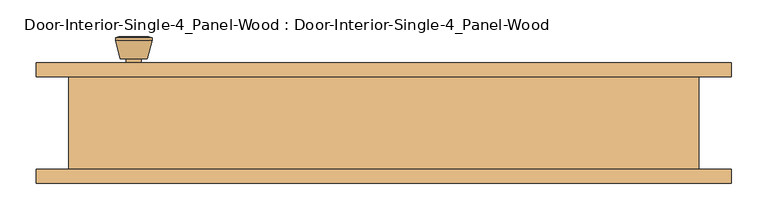
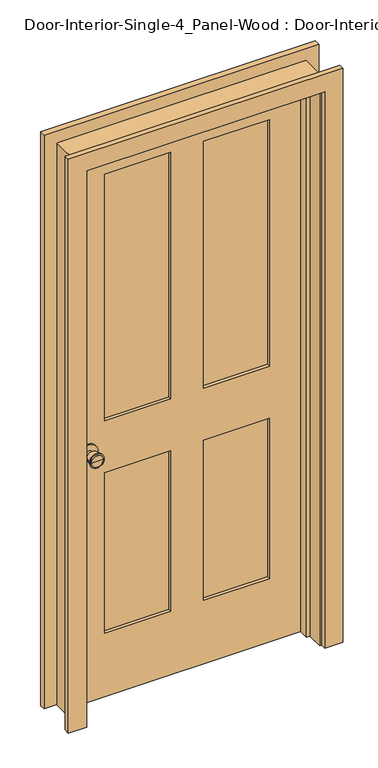
"""IFC4 building model written with IfcOpenShell, lengths in millimetres: door geometry, Door-Interior-Single-4_Panel-Wood : Door-Interior-Single-4_Panel-Wood."""

from ifc_helpers import new_model, si_unit, point, frame, frame_2d, origin, place, context, project, spatial, polyline, circle_curve, trimmed, segment, composite_curve, outline, extrude, faceted_brep, source, transform, mapped, element, save
from ifc_brep_helpers import plane_surface, cylinder_surface, revolved_surface, advanced_brep


def door_interior_single_4_panel_wood_door_interior_single_4_d89ef9d3(model_context):
    return source(origin(), model_context, "Body", "SolidModel", [
        advanced_brep(
        [(-342.9, 19.4, 914.4), (-332.9, 19.4, 914.4), (-352.9, 19.4, 914.4), (-322.4241324, -29.6, 914.4), (-342.9, -29.6, 914.4), (-363.3758676, -29.6, 914.4), (-317.9, -27.7721319, 914.4), (-367.9, -27.7721319, 914.4), (-317.9, -24.3084537, 914.4), (-367.9, -24.3084537, 914.4), (-324.263764, 0.4, 914.4), (-361.536236, 0.4, 914.4), (-332.9, 0.4, 914.4), (-352.9, 0.4, 914.4)],
        [
            (0, 1),
            (1, 2, circle_curve(frame((-342.9, 19.4, 914.4), z_axis=(0.0, 1.0, 0.0), x_axis=(-1.0, 0.0, 0.0)), 10.0)),
            (2, 0),
            (2, 1, circle_curve(frame((-342.9, 19.4, 914.4), z_axis=(0.0, 1.0, 0.0), x_axis=(-1.0, 0.0, 0.0)), 10.0)),
            (3, 4),
            (4, 5),
            (5, 3, circle_curve(frame((-342.9, -29.6, 914.4), z_axis=(0.0, -1.0, 0.0), x_axis=(-1.0, 0.0, 0.0)), 20.4758676)),
            (3, 5, circle_curve(frame((-342.9, -29.6, 914.4), z_axis=(0.0, -1.0, 0.0), x_axis=(-1.0, 0.0, 0.0)), 20.4758676)),
            (6, 3),
            (5, 7),
            (7, 6, circle_curve(frame((-342.9, -27.7721319, 914.4), z_axis=(0.0, -1.0, 0.0), x_axis=(-1.0, 0.0, 0.0)), 25.0)),
            (6, 7, circle_curve(frame((-342.9, -27.7721319, 914.4), z_axis=(0.0, -1.0, 0.0), x_axis=(-1.0, 0.0, 0.0)), 25.0)),
            (8, 6),
            (7, 9),
            (9, 8, circle_curve(frame((-342.9, -24.3084537, 914.4), z_axis=(0.0, -1.0, 0.0), x_axis=(-1.0, 0.0, 0.0)), 25.0)),
            (8, 9, circle_curve(frame((-342.9, -24.3084537, 914.4), z_axis=(0.0, -1.0, 0.0), x_axis=(-1.0, 0.0, 0.0)), 25.0)),
            (10, 8),
            (9, 11),
            (11, 10, circle_curve(frame((-342.9, 0.4, 914.4), z_axis=(0.0, -1.0, 0.0), x_axis=(-1.0, 0.0, 0.0)), 18.636236)),
            (10, 11, circle_curve(frame((-342.9, 0.4, 914.4), z_axis=(0.0, -1.0, 0.0), x_axis=(-1.0, 0.0, 0.0)), 18.636236)),
            (12, 10),
            (11, 13),
            (13, 12, circle_curve(frame((-342.9, 0.4, 914.4), z_axis=(0.0, -1.0, 0.0), x_axis=(-1.0, 0.0, 0.0)), 10.0)),
            (12, 13, circle_curve(frame((-342.9, 0.4, 914.4), z_axis=(0.0, -1.0, 0.0), x_axis=(-1.0, 0.0, 0.0)), 10.0)),
            (1, 12),
            (13, 2),
        ],
        [
            plane_surface(frame((-342.9, 19.4, 914.4), z_axis=(0.0, 1.0, 0.0), x_axis=(-1.0, 0.0, 0.0))),
            plane_surface(frame((-342.9, -29.6, 914.4), z_axis=(0.0, -1.0, 0.0), x_axis=(-1.0, 0.0, 0.0))),
            revolved_surface(polyline([(-363.3758676, -29.6, 914.4), (-367.9, -27.7721319, 914.4)]), (-342.9, 19.4, 914.4), (0.0, 1.0, 0.0)),
            cylinder_surface(frame((-342.9, 19.4, 914.4), z_axis=(0.0, 1.0, 0.0), x_axis=(-1.0, 0.0, 0.0)), 25.0),
            revolved_surface(polyline([(-367.9, -24.3084537, 914.4), (-361.536236, 0.4, 914.4)]), (-342.9, 19.4, 914.4), (0.0, 1.0, 0.0)),
            plane_surface(frame((-342.9, 0.4, 914.4), z_axis=(0.0, 1.0, 0.0), x_axis=(-1.0, 0.0, 0.0))),
            cylinder_surface(frame((-342.9, 19.4, 914.4), z_axis=(0.0, 1.0, 0.0), x_axis=(-1.0, 0.0, 0.0)), 10.0),
        ],
        [
            (0, [[1, 2, 3]]),
            (0, [[-3, 4, -1]]),
            (1, [[5, 6, 7]]),
            (1, [[-6, -5, 8]]),
            (2, [[9, -7, 10, 11]]),
            (2, [[-10, -8, -9, 12]]),
            (3, [[13, -11, 14, 15]]),
            (3, [[-14, -12, -13, 16]]),
            (4, [[17, -15, 18, 19]]),
            (4, [[-18, -16, -17, 20]]),
            (5, [[21, -19, 22, 23]]),
            (5, [[-22, -20, -21, 24]]),
            (6, [[25, -23, 26, -2]]),
            (6, [[-26, -24, -25, -4]]),
        ],
    ),
        extrude(outline(composite_curve([segment(trimmed(circle_curve(frame_2d((914.4, -342.9)), 30.0), [point((914.4, -372.9))], [point((914.4, -312.9))], False, "CARTESIAN"), True, "CONTINUOUS"), segment(trimmed(circle_curve(frame_2d((914.4, -342.9)), 30.0), [point((914.4, -312.9))], [point((914.4, -372.9))], False, "CARTESIAN"), True, "CONTINUOUS")], self_intersect=False)), frame((0.0, 19.4, 0.0), z_axis=(0.0, 1.0, 0.0), x_axis=(0.0, 0.0, 1.0)), (0.0, 0.0, 1.0), 6.0),
        advanced_brep(
        [(-342.9, 66.325, 914.4), (-352.9, 66.325, 914.4), (-332.9, 66.325, 914.4), (-322.4241324, 115.325, 914.4), (-363.3758676, 115.325, 914.4), (-342.9, 115.325, 914.4), (-317.9, 113.4971319, 914.4), (-367.9, 113.4971319, 914.4), (-317.9, 110.0334537, 914.4), (-367.9, 110.0334537, 914.4), (-324.263764, 85.325, 914.4), (-361.536236, 85.325, 914.4), (-332.9, 85.325, 914.4), (-352.9, 85.325, 914.4)],
        [
            (0, 1),
            (1, 2, circle_curve(frame((-342.9, 66.325, 914.4), z_axis=(0.0, -1.0, 0.0), x_axis=(-1.0, 0.0, 0.0)), 10.0)),
            (2, 0),
            (2, 1, circle_curve(frame((-342.9, 66.325, 914.4), z_axis=(0.0, -1.0, 0.0), x_axis=(-1.0, 0.0, 0.0)), 10.0)),
            (3, 4, circle_curve(frame((-342.9, 115.325, 914.4), z_axis=(0.0, 1.0, 0.0), x_axis=(-1.0, 0.0, 0.0)), 20.4758676)),
            (4, 5),
            (5, 3),
            (4, 3, circle_curve(frame((-342.9, 115.325, 914.4), z_axis=(0.0, 1.0, 0.0), x_axis=(-1.0, 0.0, 0.0)), 20.4758676)),
            (6, 7, circle_curve(frame((-342.9, 113.4971319, 914.4), z_axis=(0.0, 1.0, 0.0), x_axis=(-1.0, 0.0, 0.0)), 25.0)),
            (7, 4),
            (3, 6),
            (7, 6, circle_curve(frame((-342.9, 113.4971319, 914.4), z_axis=(0.0, 1.0, 0.0), x_axis=(-1.0, 0.0, 0.0)), 25.0)),
            (8, 9, circle_curve(frame((-342.9, 110.0334537, 914.4), z_axis=(0.0, 1.0, 0.0), x_axis=(-1.0, 0.0, 0.0)), 25.0)),
            (9, 7),
            (6, 8),
            (9, 8, circle_curve(frame((-342.9, 110.0334537, 914.4), z_axis=(0.0, 1.0, 0.0), x_axis=(-1.0, 0.0, 0.0)), 25.0)),
            (10, 11, circle_curve(frame((-342.9, 85.325, 914.4), z_axis=(0.0, 1.0, 0.0), x_axis=(-1.0, 0.0, 0.0)), 18.636236)),
            (11, 9),
            (8, 10),
            (11, 10, circle_curve(frame((-342.9, 85.325, 914.4), z_axis=(0.0, 1.0, 0.0), x_axis=(-1.0, 0.0, 0.0)), 18.636236)),
            (12, 13, circle_curve(frame((-342.9, 85.325, 914.4), z_axis=(0.0, 1.0, 0.0), x_axis=(-1.0, 0.0, 0.0)), 10.0)),
            (13, 11),
            (10, 12),
            (13, 12, circle_curve(frame((-342.9, 85.325, 914.4), z_axis=(0.0, 1.0, 0.0), x_axis=(-1.0, 0.0, 0.0)), 10.0)),
            (1, 13),
            (12, 2),
        ],
        [
            plane_surface(frame((-342.9, 66.325, 914.4), z_axis=(0.0, -1.0, 0.0), x_axis=(-1.0, 0.0, 0.0))),
            plane_surface(frame((-342.9, 115.325, 914.4), z_axis=(0.0, 1.0, 0.0), x_axis=(-1.0, 0.0, 0.0))),
            revolved_surface(polyline([(-363.3758676, 115.325, 914.4), (-367.9, 113.4971319, 914.4)]), (-342.9, 66.325, 914.4), (0.0, -1.0, 0.0)),
            cylinder_surface(frame((-342.9, 66.325, 914.4), z_axis=(0.0, -1.0, 0.0), x_axis=(-1.0, 0.0, 0.0)), 25.0),
            revolved_surface(polyline([(-367.9, 110.0334537, 914.4), (-361.536236, 85.325, 914.4)]), (-342.9, 66.325, 914.4), (0.0, -1.0, 0.0)),
            plane_surface(frame((-342.9, 85.325, 914.4), z_axis=(0.0, -1.0, 0.0), x_axis=(-1.0, 0.0, 0.0))),
            cylinder_surface(frame((-342.9, 66.325, 914.4), z_axis=(0.0, -1.0, 0.0), x_axis=(-1.0, 0.0, 0.0)), 10.0),
        ],
        [
            (0, [[1, 2, 3]]),
            (0, [[-3, 4, -1]]),
            (1, [[5, 6, 7]]),
            (1, [[8, -7, -6]]),
            (2, [[9, 10, -5, 11]]),
            (2, [[12, -11, -8, -10]]),
            (3, [[13, 14, -9, 15]]),
            (3, [[16, -15, -12, -14]]),
            (4, [[17, 18, -13, 19]]),
            (4, [[20, -19, -16, -18]]),
            (5, [[21, 22, -17, 23]]),
            (5, [[24, -23, -20, -22]]),
            (6, [[-2, 25, -21, 26]]),
            (6, [[-4, -26, -24, -25]]),
        ],
    ),
        extrude(outline(composite_curve([segment(trimmed(circle_curve(frame_2d((914.4, -342.9)), 30.0), [point((914.4, -372.9))], [point((914.4, -312.9))], False, "CARTESIAN"), True, "CONTINUOUS"), segment(trimmed(circle_curve(frame_2d((914.4, -342.9)), 30.0), [point((914.4, -312.9))], [point((914.4, -372.9))], False, "CARTESIAN"), True, "CONTINUOUS")], self_intersect=False)), frame((0.0, 60.325, 0.0), z_axis=(0.0, 1.0, 0.0), x_axis=(0.0, 0.0, 1.0)), (0.0, 0.0, 1.0), 6.0),
        faceted_brep([(431.8, 60.325, 0.0), (431.8, -66.675, 0.0), (406.4, -66.675, 0.0), (406.4, -9.525, 0.0), (393.7, -9.525, 0.0), (393.7, 25.4, 0.0), (406.4, 25.4, 0.0), (406.4, 60.325, 0.0), (431.8, 60.325, 2057.4), (431.8, -66.675, 2057.4), (-431.8, -66.675, 2057.4), (-431.8, -66.675, 0.0), (-406.4, -66.675, 0.0), (-406.4, -66.675, 2032.0), (406.4, -66.675, 2032.0), (406.4, -9.525, 2032.0), (-406.4, -9.525, 2032.0), (-406.4, -9.525, 0.0), (-393.7, -9.525, 0.0), (-393.7, -9.525, 2019.3), (393.7, -9.525, 2019.3), (393.7, 25.4, 2019.3), (-393.7, 25.4, 2019.3), (-393.7, 25.4, 0.0), (-406.4, 25.4, 0.0), (-406.4, 25.4, 2032.0), (406.4, 25.4, 2032.0), (406.4, 60.325, 2032.0), (-406.4, 60.325, 2032.0), (-406.4, 60.325, 0.0), (-431.8, 60.325, 0.0), (-431.8, 60.325, 2057.4)], [[[0, 1, 2, 3, 4, 5, 6, 7]], [[1, 0, 8, 9]], [[2, 1, 9, 10, 11, 12, 13, 14]], [[3, 2, 14, 15]], [[4, 3, 15, 16, 17, 18, 19, 20]], [[5, 4, 20, 21]], [[6, 5, 21, 22, 23, 24, 25, 26]], [[7, 6, 26, 27]], [[0, 7, 27, 28, 29, 30, 31, 8]], [[9, 8, 31, 10]], [[15, 14, 13, 16]], [[21, 20, 19, 22]], [[27, 26, 25, 28]], [[30, 29, 24, 23, 18, 17, 12, 11]], [[10, 31, 30, 11]], [[16, 13, 12, 17]], [[22, 19, 18, 23]], [[28, 25, 24, 29]]]),
        extrude(outline(polyline([(2032.0, -406.4), (0.0, -406.4), (0.0, 406.4), (2032.0, 406.4), (2032.0, -406.4)]), holes=[polyline([(1912.9375, 57.15), (1912.9375, 285.75), (1009.65, 285.75), (1009.65, 57.15), (1912.9375, 57.15)]), polyline([(1009.65, -57.15), (1009.65, -285.75), (1912.9375, -285.75), (1912.9375, -57.15), (1009.65, -57.15)]), polyline([(819.15, 57.15), (819.15, 285.75), (231.775, 285.75), (231.775, 57.15), (819.15, 57.15)]), polyline([(231.775, -57.15), (231.775, -285.75), (819.15, -285.75), (819.15, -57.15), (231.775, -57.15)])]), frame((0.0, 25.4, 0.0), z_axis=(0.0, 1.0, 0.0), x_axis=(0.0, 0.0, 1.0)), (0.0, 0.0, 1.0), 34.925),
        extrude(outline(polyline([(285.75, 37.0416667), (57.15, 37.0416667), (57.15, 48.6833333), (285.75, 48.6833333), (285.75, 37.0416667)])), frame((0.0, 0.0, 1009.65), z_axis=(0.0, 0.0, 1.0), x_axis=(1.0, 0.0, 0.0)), (0.0, 0.0, 1.0), 903.2875),
        extrude(outline(polyline([(-57.15, 37.0416667), (-285.75, 37.0416667), (-285.75, 48.6833333), (-57.15, 48.6833333), (-57.15, 37.0416667)])), frame((0.0, 0.0, 1009.65), z_axis=(0.0, 0.0, 1.0), x_axis=(1.0, 0.0, 0.0)), (0.0, 0.0, 1.0), 903.2875),
        extrude(outline(polyline([(285.75, 37.0416667), (57.15, 37.0416667), (57.15, 48.6833333), (285.75, 48.6833333), (285.75, 37.0416667)])), frame((0.0, 0.0, 231.775), z_axis=(0.0, 0.0, 1.0), x_axis=(1.0, 0.0, 0.0)), (0.0, 0.0, 1.0), 587.375),
        extrude(outline(polyline([(-57.15, 37.0416667), (-285.75, 37.0416667), (-285.75, 48.6833333), (-57.15, 48.6833333), (-57.15, 37.0416667)])), frame((0.0, 0.0, 231.775), z_axis=(0.0, 0.0, 1.0), x_axis=(1.0, 0.0, 0.0)), (0.0, 0.0, 1.0), 587.375),
        extrude(outline(polyline([(0.0, 412.75), (0.0, 476.25), (2101.85, 476.25), (2101.85, -476.25), (0.0, -476.25), (0.0, -412.75), (2038.35, -412.75), (2038.35, 412.75), (0.0, 412.75)])), frame((0.0, 60.325, 0.0), z_axis=(0.0, 1.0, 0.0), x_axis=(0.0, 0.0, 1.0)), (0.0, 0.0, 1.0), 19.05),
        extrude(outline(polyline([(0.0, 412.75), (0.0, 476.25), (2101.85, 476.25), (2101.85, -476.25), (0.0, -476.25), (0.0, -412.75), (2038.35, -412.75), (2038.35, 412.75), (0.0, 412.75)])), frame((0.0, -85.725, 0.0), z_axis=(0.0, 1.0, 0.0), x_axis=(0.0, 0.0, 1.0)), (0.0, 0.0, 1.0), 19.05),
    ])


if __name__ == "__main__":
    model = new_model("IFC4")
    model_context = context("Model", 3, world=origin())
    ifc_project = project(units=[si_unit("LENGTHUNIT", "METRE", prefix="MILLI")], contexts=[model_context])
    site = spatial("IfcSite", under=ifc_project)
    building = spatial("IfcBuilding", under=site)
    placement = place(None, origin())
    door_interior_single_4_panel_wood_door_interior_single_4_shape = door_interior_single_4_panel_wood_door_interior_single_4_d89ef9d3(model_context)
    element("IfcDoor", 1, ObjectType="Door-Interior-Single-4_Panel-Wood : Door-Interior-Single-4_Panel-Wood", at=placement, inside=building, context=model_context, shape_type="MappedRepresentation", body=[
        mapped(door_interior_single_4_panel_wood_door_interior_single_4_shape, transform((0.0, 0.0, 0.0), x_axis=(1.0, 0.0, 0.0), y_axis=(0.0, 1.0, 0.0), z_axis=(0.0, 0.0, 1.0))),
    ])
    save(model, "model.ifc")

# Revit data of these elements
# Type "Door-Interior-Single-4_Panel-Wood : Door-Interior-Single-4_Panel-Wood"
#   Type Mark = "9"
#   Assembly Code = "C1020300"
#   Analytic Construction = "Wooden"
#   Top Rail = 0' - 4 11/16"
#   Thickness = 0' - 1 3/8"
#   Thermal Resistance (R) = 2.5876 (h·ft²·°F)/BTU
#   Swing Angle [instance default] = 90.00°
#   Stiles = 0' - 4 3/4"
#   Rough Width = 2' - 10"
#   Rough Height = 6' - 9"
#   Mullion = 0' - 4 1/2"
#   Lock Rail = 0' - 7 1/2"
#   Height = 6' - 8"
#   Width = 2' - 8"
#   Heat Transfer Coefficient (U) = 0.3865 BTU/(h·ft²·°F)
#   Bottom Rail = 0' - 9 1/8"
#   Trim Material = Cherry
#   Panel Material = Cherry
#   Frame Material = Cherry
#   Door Handle Material = Aluminum
#   Visual Light Transmittance = 0
#   Solar Heat Gain Coefficient = 0
#   Wall Closure = (empty or 0)
#   Function = (empty or 0)
# Element 1 (IfcDoor, "Door-Interior-Single-4_Panel-Wood : Door-Interior-Single-4_Panel-Wood")
#   Materials on its faces: "Cherry", "Aluminum"
# Materials
#   "Cherry": class "Wood", colour RGB 226 177 128, transparency 0, Description = "Prunus Serotina", Cost = 0
#   "Aluminum": class "Metal", colour RGB 247 247 247, transparency 0, Description = "Aluminum 6061", Cost = 0
